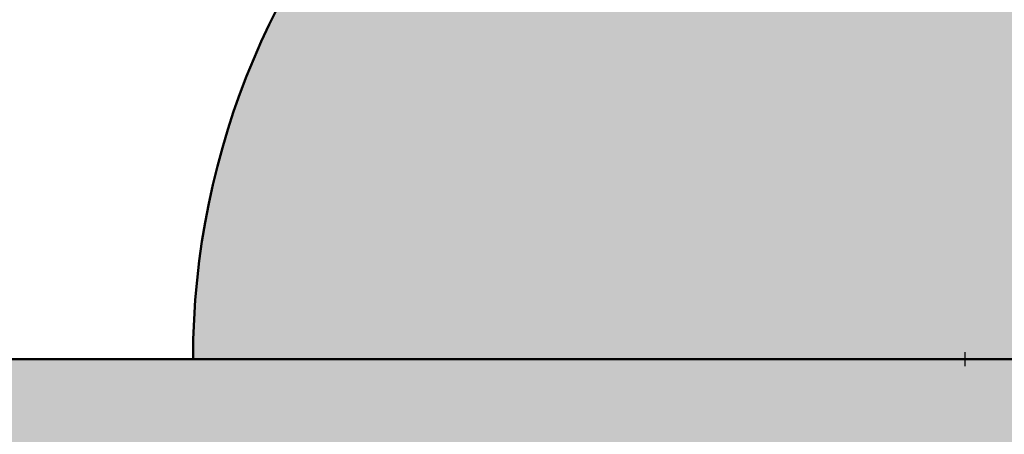
# Model space of a CAD drawing. Units: millimetres. Extents: x 0 to 2267, y 0 to 1823.
# Tile 14 of 256: x 1518.68 to 1531.44, y 1116.44 to 1121.82. Entities that reach past the tile are written whole.
import ezdxf

# ---------------------------------------------------------------- set-up
doc = ezdxf.new("R2010")
doc.units = ezdxf.units.MM
doc.header["$MEASUREMENT"] = 0
for name, color, linetype, lineweight in [('M-DIMS', 2, 'Continuous', 25), ('M-HATC', 252, 'Continuous', 18), ('M-OUTL', 7, 'Continuous', 50)]:
    doc.layers.add(name, color=color, linetype=linetype, lineweight=lineweight)
doc.styles.get("Standard").update_dxf_attribs({"font": 'arial.ttf'})
doc.dimstyles.get("Standard").update_dxf_attribs({"dimtxt": 7, "dimasz": 4, "dimexe": 0.18, "dimexo": 0.0625, "dimgap": 0.09, "dimtad": 0, "dimdec": 0, "dimzin": 0, "dimdsep": 46, "dimtxsty": 'Standard', "dimcen": 0.09, "dimadec": 0, "dimazin": 0, "dimtfac": 1, "dimtdec": 0, "dimtofl": 0, "dimtmove": 0, "dimatfit": 3, "dimfxl": 1, "dimtolj": 1, "dimtzin": 0, "dimarcsym": 0})

# ---------------------------------------------------------------- blocks, each defined once
blk = doc.blocks.new('*D28')
at = {"layer": 'Defpoints', "color": 0, "transparency": 16777216}
for p in [(1523.858, 1124.488), (1530.929, 1117.417)]:
    blk.add_point(p, dxfattribs=at)
at = {"layer": 'M-DIMS', "color": 0, "lineweight": -2, "transparency": 16777216}
for p, q in [((1518.201, 1130.145), (1521.029, 1127.317)), ((1530.839, 1117.417), (1531.019, 1117.417)), ((1530.929, 1117.327), (1530.929, 1117.507))]:
    blk.add_line(p, q, dxfattribs=at)
at = {"layer": 'M-DIMS', "color": 0, "transparency": 16777216}
blk.add_solid([(1521.501, 1127.788), (1520.558, 1126.845), (1523.858, 1124.488)], dxfattribs=at)
at = {"layer": 'M-DIMS', "color": 0, "transparency": 16777216, "insert": (1504.949, 1143.397), "char_height": 7, "attachment_point": 5, "rotation": 314.9998}
blk.add_mtext('\\A1;27X R10', dxfattribs=at)

msp = doc.modelspace()

# ---------------------------------------------------------------- hatches: boundary and pattern name
at = {"layer": 'M-HATC'}
h = msp.add_hatch(color=256, dxfattribs=at)
h.dxf.hatch_style = 1
h.paths.add_polyline_path([(2065.771, 1618.062, 0.236068), (2055.771, 1638.062), (1381.087, 1638.062, 0.236068), (1371.087, 1618.062), (1371.087, 1603.062), (2055.771, 1603.062), (2065.771, 1603.062)])
h.paths.add_polyline_path([(2062.772, 1550.296), (2062.772, 1560.296), (1374.086, 1560.296), (1374.086, 1550.296), (1374.086, 1540.296), (1384.086, 1540.296), (1389.086, 1540.296), (2062.772, 1540.296)])
h.paths.add_polyline_path([(1930.929, 1282.766), (1505.929, 1282.766), (1587.628, 1235.597, 0.131652), (1600.128, 1232.247), (1836.73, 1232.247, 0.131652), (1849.23, 1235.597)])
h.paths.add_polyline_path([(1930.929, 1117.417), (1905.929, 1117.417), (1505.929, 1117.417), (1505.929, 1077.417), (1930.929, 1077.417)])
h = msp.add_hatch(color=256, dxfattribs=at)
h.dxf.hatch_style = 1
h.paths.add_polyline_path([(2055.771, 1603.062), (1381.087, 1603.062), (1381.087, 1598.062), (2055.771, 1598.062)])
h.paths.add_polyline_path([(2055.771, 1598.062), (1381.087, 1598.062), (1381.087, 1593.062), (2055.771, 1593.062)])
h.paths.add_polyline_path([(2051.307, 1536.761), (1385.55, 1536.761), (1385.55, 1526.761), (1387.55, 1526.761), (1388.537, 1525.053), (1385.332, 1521.233), (1385.332, 1521.223), (2050.254, 1522.749), (2048.321, 1525.053), (2049.307, 1526.761), (2051.307, 1526.761)])
edge = h.paths.add_edge_path()
edge.add_arc((1847.535, 1379.149), 135, 222.60306, 222.89085, ccw=False)
edge.add_line((1748.166, 1287.766), (1683.092, 1287.766))
edge.add_arc((1583.724, 1379.149), 135, 317.10915, 317.39694, ccw=False)
edge.add_arc((1678.969, 1290.671), 5, 222.8909, 317.1091, ccw=False)
edge.add_arc((1774.213, 1379.149), 135, 222.60306, 222.89085, ccw=False)
edge.add_line((1674.845, 1287.766), (1609.771, 1287.766))
edge.add_arc((1510.403, 1379.149), 135, 317.10915, 317.39694, ccw=False)
edge.add_arc((1605.647, 1290.671), 5, 222.8909, 317.1091, ccw=False)
edge.add_arc((1700.892, 1379.149), 135, 222.60306, 222.89085, ccw=False)
edge.add_line((1601.524, 1287.766), (1536.45, 1287.766))
edge.add_arc((1437.081, 1379.149), 135, 317.10915, 317.39694, ccw=False)
edge.add_arc((1532.326, 1290.671), 5, 222.8909, 317.1091, ccw=False)
edge.add_arc((1627.571, 1379.149), 135, 222.60306, 222.89085, ccw=False)
edge.add_line((1528.203, 1287.766), (1505.929, 1287.766))
edge.add_spline(control_points=[(1505.929, 1287.766), (1504.262, 1287.766), (1504.262, 1282.766), (1505.929, 1282.766)], knot_values=[0, 0, 0, 0, 5, 5, 5, 5], degree=3, periodic=0)
edge.add_line((1505.929, 1282.766), (1930.929, 1282.766))
edge.add_spline(control_points=[(1930.929, 1282.766), (1932.596, 1282.766), (1932.596, 1287.766), (1930.929, 1287.766)], knot_values=[0, 0, 0, 0, 5, 5, 5, 5], degree=3, periodic=0)
edge.add_line((1930.929, 1287.766), (1903.056, 1287.766))
edge.add_arc((1803.688, 1379.149), 135, 317.10915, 317.39694, ccw=False)
edge.add_arc((1898.932, 1290.671), 5, 222.8909, 317.1091, ccw=False)
edge.add_arc((1994.177, 1379.149), 135, 222.60306, 222.89085, ccw=False)
edge.add_line((1894.809, 1287.766), (1829.735, 1287.766))
edge.add_arc((1730.366, 1379.149), 135, 317.10915, 317.39694, ccw=False)
edge.add_arc((1825.611, 1290.671), 5, 222.8909, 317.1091, ccw=False)
edge.add_arc((1920.856, 1379.149), 135, 222.60306, 222.89085, ccw=False)
edge.add_line((1821.487, 1287.766), (1756.413, 1287.766))
edge.add_arc((1657.045, 1379.149), 135, 317.10915, 317.39694, ccw=False)
edge.add_arc((1752.29, 1290.671), 5, 222.8909, 317.1091, ccw=False)
edge = h.paths.add_edge_path()
edge.add_spline(control_points=[(1843.429, 1227.247), (1845.096, 1227.247), (1845.096, 1232.247), (1843.429, 1232.247)], knot_values=[0, 0, 0, 0, 5, 5, 5, 5], degree=3, periodic=0)
edge.add_line((1843.429, 1232.247), (1593.429, 1232.247))
edge.add_spline(control_points=[(1593.429, 1232.247), (1591.762, 1232.247), (1591.762, 1227.247), (1593.429, 1227.247)], knot_values=[0, 0, 0, 0, 5, 5, 5, 5], degree=3, periodic=0)
edge.add_line((1593.429, 1227.247), (1843.429, 1227.247))
h.paths.add_polyline_path([(1905.929, 1127.417), (1530.929, 1127.417, 0.414214), (1520.929, 1117.417), (1530.929, 1117.417), (1915.929, 1117.417, 0.414214)])
edge = h.paths.add_edge_path()
edge.add_arc((1397.086, 1498.408), 12.73, 90.7821, 190.8787, ccw=False)
edge.add_line((1396.912, 1511.136), (1428.01, 1511.349))
edge.add_line((1428.01, 1511.349), (1433.01, 1511.349))
edge.add_line((1433.01, 1511.349), (1434.439, 1511.349))
edge.add_arc((1419.474, 1498.08), 20, 41.561, 74.0821)
edge.add_line((1424.959, 1517.314), (1399.935, 1517.256))
edge.add_spline(control_points=[(1399.931, 1517.256), (1399.884, 1517.213), (1399.833, 1517.169), (1399.777, 1517.124)], knot_values=[11.567499, 11.567499, 11.567499, 11.567499, 11.814249, 11.814249, 11.814249, 11.814249], degree=3, periodic=0)
edge.add_spline(control_points=[(1399.633, 1517.01), (1399.583, 1516.972), (1399.531, 1516.934), (1399.476, 1516.895)], knot_values=[11.167718, 11.167718, 11.167718, 11.167718, 11.365188, 11.365188, 11.365188, 11.365188], degree=3, periodic=0)
edge.add_spline(control_points=[(1399.34, 1516.8), (1399.151, 1516.672), (1398.938, 1516.538), (1398.704, 1516.399)], knot_values=[10.376405, 10.376405, 10.376405, 10.376405, 11.00994, 11.00994, 11.00994, 11.00994], degree=3, periodic=0)
edge.add_spline(control_points=[(1398.657, 1516.372), (1398.579, 1516.326), (1398.498, 1516.28), (1398.415, 1516.233)], knot_values=[10.125175, 10.125175, 10.125175, 10.125175, 10.334406, 10.334406, 10.334406, 10.334406], degree=3, periodic=0)
edge.add_spline(control_points=[(1398.264, 1516.149), (1398.196, 1516.111), (1398.126, 1516.073), (1398.055, 1516.035)], knot_values=[9.832246, 9.832246, 9.832246, 9.832246, 9.999658, 9.999658, 9.999658, 9.999658], degree=3, periodic=0)
edge.add_spline(control_points=[(1397.999, 1516.005), (1397.731, 1515.862), (1397.446, 1515.717), (1397.147, 1515.571)], knot_values=[9.161808, 9.161808, 9.161808, 9.161808, 9.787769, 9.787769, 9.787769, 9.787769], degree=3, periodic=0)
edge.add_spline(control_points=[(1397.147, 1515.571), (1396.842, 1515.423), (1396.522, 1515.274), (1396.191, 1515.126)], knot_values=[8.524455, 8.524455, 8.524455, 8.524455, 9.161808, 9.161808, 9.161808, 9.161808], degree=3, periodic=0)
edge.add_spline(control_points=[(1396.078, 1515.076), (1395.985, 1515.035), (1395.892, 1514.994), (1395.798, 1514.953)], knot_values=[8.275193, 8.275193, 8.275193, 8.275193, 8.451726, 8.451726, 8.451726, 8.451726], degree=3, periodic=0)
edge.add_spline(control_points=[(1395.602, 1514.869), (1395.5, 1514.826), (1395.397, 1514.782), (1395.293, 1514.739)], knot_values=[7.962917, 7.962917, 7.962917, 7.962917, 8.152764, 8.152764, 8.152764, 8.152764], degree=3, periodic=0)
edge.add_spline(control_points=[(1395.212, 1514.706), (1394.828, 1514.547), (1394.435, 1514.393), (1394.036, 1514.244)], knot_values=[7.21254, 7.21254, 7.21254, 7.21254, 7.913148, 7.913148, 7.913148, 7.913148], degree=3, periodic=0)
edge.add_spline(control_points=[(1394.036, 1514.244), (1393.708, 1514.121), (1393.375, 1514.003), (1393.043, 1513.889)], knot_values=[6.633733, 6.633733, 6.633733, 6.633733, 7.21254, 7.21254, 7.21254, 7.21254], degree=3, periodic=0)
edge.add_spline(control_points=[(1392.821, 1513.815), (1392.72, 1513.781), (1392.618, 1513.748), (1392.517, 1513.715)], knot_values=[6.328796, 6.328796, 6.328796, 6.328796, 6.505493, 6.505493, 6.505493, 6.505493], degree=3, periodic=0)
edge.add_spline(control_points=[(1392.517, 1513.715), (1392.319, 1513.652), (1392.121, 1513.59), (1391.924, 1513.531)], knot_values=[5.984605, 5.984605, 5.984605, 5.984605, 6.328796, 6.328796, 6.328796, 6.328796], degree=3, periodic=0)
edge.add_spline(control_points=[(1391.792, 1513.491), (1391.312, 1513.35), (1390.838, 1513.224), (1390.378, 1513.117)], knot_values=[5.066697, 5.066697, 5.066697, 5.066697, 5.907055, 5.907055, 5.907055, 5.907055], degree=3, periodic=0)
edge.add_spline(control_points=[(1390.378, 1513.117), (1390.18, 1513.071), (1389.984, 1513.028), (1389.791, 1512.99)], knot_values=[4.70367, 4.70367, 4.70367, 4.70367, 5.066695, 5.066695, 5.066695, 5.066695], degree=3, periodic=0)
edge.add_spline(control_points=[(1389.422, 1512.92), (1389.246, 1512.889), (1389.073, 1512.862), (1388.904, 1512.838)], knot_values=[4.130571, 4.130571, 4.130571, 4.130571, 4.469816, 4.469816, 4.469816, 4.469816], degree=3, periodic=0)
edge.add_spline(control_points=[(1388.904, 1512.838), (1388.591, 1512.795), (1388.291, 1512.764), (1388.007, 1512.749)], knot_values=[3.504031, 3.504031, 3.504031, 3.504031, 4.130571, 4.130571, 4.130571, 4.130571], degree=3, periodic=0)
edge.add_spline(control_points=[(1387.936, 1512.746), (1387.854, 1512.742), (1387.773, 1512.74), (1387.694, 1512.739)], knot_values=[3.268866, 3.268866, 3.268866, 3.268866, 3.451164, 3.451164, 3.451164, 3.451164], degree=3, periodic=0)
edge.add_spline(control_points=[(1387.335, 1512.744), (1387.208, 1512.75), (1387.085, 1512.76), (1386.967, 1512.774)], knot_values=[2.670686, 2.670686, 2.670686, 2.670686, 2.984, 2.984, 2.984, 2.984], degree=3, periodic=0)
edge.add_spline(control_points=[(1386.833, 1512.792), (1386.821, 1512.794), (1386.809, 1512.796), (1386.797, 1512.798)], knot_values=[2.516981, 2.516981, 2.516981, 2.516981, 2.549528, 2.549528, 2.549528, 2.549528], degree=3, periodic=0)
edge.add_spline(control_points=[(1386.453, 1512.873), (1386.426, 1512.881), (1386.399, 1512.889), (1386.373, 1512.897)], knot_values=[2.095869, 2.095869, 2.095869, 2.095869, 2.17941, 2.17941, 2.17941, 2.17941], degree=3, periodic=0)
edge.add_spline(control_points=[(1386.069, 1513.019), (1386.063, 1513.022), (1386.058, 1513.025), (1386.052, 1513.028)], knot_values=[1.72453, 1.72453, 1.72453, 1.72453, 1.745933, 1.745933, 1.745933, 1.745933], degree=3, periodic=0)
edge.add_arc((1399.474, 1498.08), 20, 131.8243, 180)
edge.add_arc((1630.334, 1505.548), 250.971, 181.70518, 236.42798)
edge.add_arc((1605.34, 1483.304), 218.782, 238.66083, 243.34961)
edge.add_arc((1647.091, 1510.359), 262.899, 183.12984, 237.85344, ccw=False)
h.paths.add_polyline_path([(1406.537, 1391.964, 0.149382), (1491.551, 1296.442, -0.129517)], flags=17)
edge = h.paths.add_edge_path()
edge.add_arc((2037.384, 1498.08), 20, 0, 48.2659)
edge.add_spline(control_points=[(2050.697, 1513.005), (2050.651, 1512.985), (2050.603, 1512.966), (2050.554, 1512.948)], knot_values=[1.835652, 1.835652, 1.835652, 1.835652, 2.000781, 2.000781, 2.000781, 2.000781], degree=3, periodic=0)
edge.add_spline(control_points=[(2050.462, 1512.917), (2050.479, 1512.922), (2050.496, 1512.928), (2050.513, 1512.934)], knot_values=[2.045477, 2.045477, 2.045477, 2.045477, 2.101389, 2.101389, 2.101389, 2.101389], degree=3, periodic=0)
edge.add_spline(control_points=[(2050.129, 1512.834), (2050.198, 1512.847), (2050.266, 1512.862), (2050.331, 1512.879)], knot_values=[2.237629, 2.237629, 2.237629, 2.237629, 2.435841, 2.435841, 2.435841, 2.435841], degree=3, periodic=0)
edge.add_spline(control_points=[(2050.095, 1512.828), (2050.106, 1512.83), (2050.118, 1512.832), (2050.129, 1512.834)], knot_values=[2.435841, 2.435841, 2.435841, 2.435841, 2.468321, 2.468321, 2.468321, 2.468321], degree=3, periodic=0)
edge.add_spline(control_points=[(2049.784, 1512.785), (2049.855, 1512.792), (2049.924, 1512.801), (2049.992, 1512.811)], knot_values=[2.563852, 2.563852, 2.563852, 2.563852, 2.748541, 2.748541, 2.748541, 2.748541], degree=3, periodic=0)
edge.add_spline(control_points=[(2049.405, 1512.762), (2049.536, 1512.765), (2049.663, 1512.773), (2049.784, 1512.785)], knot_values=[2.748541, 2.748541, 2.748541, 2.748541, 3.064882, 3.064882, 3.064882, 3.064882], degree=3, periodic=0)
edge.add_spline(control_points=[(2049.17, 1512.76), (2049.234, 1512.759), (2049.297, 1512.759), (2049.358, 1512.761)], knot_values=[3.102309, 3.102309, 3.102309, 3.102309, 3.2503, 3.2503, 3.2503, 3.2503], degree=3, periodic=0)
edge.add_spline(control_points=[(2048.857, 1512.769), (2048.964, 1512.764), (2049.068, 1512.761), (2049.17, 1512.76)], knot_values=[3.2503, 3.2503, 3.2503, 3.2503, 3.486069, 3.486069, 3.486069, 3.486069], degree=3, periodic=0)
edge.add_spline(control_points=[(2048.692, 1512.779), (2048.373, 1512.801), (2048.035, 1512.841), (2047.682, 1512.897)], knot_values=[3.606429, 3.606429, 3.606429, 3.606429, 4.2989, 4.2989, 4.2989, 4.2989], degree=3, periodic=0)
edge.add_spline(control_points=[(2047.682, 1512.897), (2047.546, 1512.919), (2047.408, 1512.942), (2047.268, 1512.969)], knot_values=[4.2989, 4.2989, 4.2989, 4.2989, 4.565769, 4.565769, 4.565769, 4.565769], degree=3, periodic=0)
edge.add_spline(control_points=[(2047.268, 1512.969), (2047.145, 1512.991), (2047.021, 1513.016), (2046.895, 1513.042)], knot_values=[4.565769, 4.565769, 4.565769, 4.565769, 4.799971, 4.799971, 4.799971, 4.799971], degree=3, periodic=0)
edge.add_spline(control_points=[(2046.895, 1513.042), (2046.529, 1513.119), (2046.151, 1513.209), (2045.768, 1513.311)], knot_values=[4.799971, 4.799971, 4.799971, 4.799971, 5.483718, 5.483718, 5.483718, 5.483718], degree=3, periodic=0)
edge.add_spline(control_points=[(2045.768, 1513.311), (2045.372, 1513.415), (2044.97, 1513.532), (2044.566, 1513.659)], knot_values=[5.483718, 5.483718, 5.483718, 5.483718, 6.187866, 6.187866, 6.187866, 6.187866], degree=3, periodic=0)
edge.add_spline(control_points=[(2044.566, 1513.659), (2044.415, 1513.706), (2044.263, 1513.755), (2044.112, 1513.805)], knot_values=[6.187866, 6.187866, 6.187866, 6.187866, 6.451551, 6.451551, 6.451551, 6.451551], degree=3, periodic=0)
edge.add_spline(control_points=[(2044.112, 1513.805), (2043.997, 1513.843), (2043.882, 1513.881), (2043.767, 1513.92)], knot_values=[6.451551, 6.451551, 6.451551, 6.451551, 6.651434, 6.651434, 6.651434, 6.651434], degree=3, periodic=0)
edge.add_spline(control_points=[(2043.767, 1513.92), (2043.372, 1514.055), (2042.977, 1514.198), (2042.589, 1514.346)], knot_values=[6.651434, 6.651434, 6.651434, 6.651434, 7.338879, 7.338879, 7.338879, 7.338879], degree=3, periodic=0)
edge.add_spline(control_points=[(2042.589, 1514.346), (2042.164, 1514.507), (2041.746, 1514.675), (2041.341, 1514.846)], knot_values=[7.338879, 7.338879, 7.338879, 7.338879, 8.089209, 8.089209, 8.089209, 8.089209], degree=3, periodic=0)
edge.add_spline(control_points=[(2041.341, 1514.846), (2041.103, 1514.946), (2040.869, 1515.048), (2040.64, 1515.15)], knot_values=[8.089209, 8.089209, 8.089209, 8.089209, 8.529587, 8.529587, 8.529587, 8.529587], degree=3, periodic=0)
edge.add_spline(control_points=[(2040.51, 1515.209), (2040.082, 1515.402), (2039.675, 1515.597), (2039.295, 1515.789)], knot_values=[8.613818, 8.613818, 8.613818, 8.613818, 9.44571, 9.44571, 9.44571, 9.44571], degree=3, periodic=0)
edge.add_spline(control_points=[(2039.295, 1515.789), (2039.062, 1515.907), (2038.839, 1516.025), (2038.629, 1516.14)], knot_values=[9.44571, 9.44571, 9.44571, 9.44571, 9.956404, 9.956404, 9.956404, 9.956404], degree=3, periodic=0)
edge.add_spline(control_points=[(2038.629, 1516.14), (2038.519, 1516.2), (2038.412, 1516.26), (2038.309, 1516.319)], knot_values=[9.956404, 9.956404, 9.956404, 9.956404, 10.223542, 10.223542, 10.223542, 10.223542], degree=3, periodic=0)
edge.add_spline(control_points=[(2038.309, 1516.319), (2038.214, 1516.374), (2038.122, 1516.428), (2038.033, 1516.481)], knot_values=[10.223542, 10.223542, 10.223542, 10.223542, 10.47051, 10.47051, 10.47051, 10.47051], degree=3, periodic=0)
edge.add_spline(control_points=[(2038.033, 1516.481), (2037.786, 1516.63), (2037.564, 1516.773), (2037.372, 1516.909)], knot_values=[10.47051, 10.47051, 10.47051, 10.47051, 11.15767, 11.15767, 11.15767, 11.15767], degree=3, periodic=0)
edge.add_spline(control_points=[(2037.372, 1516.909), (2037.279, 1516.975), (2037.193, 1517.04), (2037.114, 1517.102)], knot_values=[11.15767, 11.15767, 11.15767, 11.15767, 11.49227, 11.49227, 11.49227, 11.49227], degree=3, periodic=0)
edge.add_spline(control_points=[(2036.856, 1517.326), (2036.915, 1517.269), (2036.981, 1517.21), (2037.056, 1517.149)], knot_values=[11.577341, 11.577341, 11.577341, 11.577341, 11.91035, 11.91035, 11.91035, 11.91035], degree=3, periodic=0)
edge.add_spline(control_points=[(2036.807, 1517.375), (2036.823, 1517.359), (2036.839, 1517.342), (2036.856, 1517.326)], knot_values=[11.91035, 11.91035, 11.91035, 11.91035, 12.007402, 12.007402, 12.007402, 12.007402], degree=3, periodic=0)
edge.add_spline(control_points=[(2036.702, 1517.494), (2036.71, 1517.483), (2036.72, 1517.472), (2036.729, 1517.461)], knot_values=[12.184155, 12.184155, 12.184155, 12.184155, 12.255409, 12.255409, 12.255409, 12.255409], degree=3, periodic=0)
edge.add_spline(control_points=[(2036.616, 1517.621), (2036.62, 1517.613), (2036.624, 1517.606), (2036.629, 1517.598)], knot_values=[12.487913, 12.487913, 12.487913, 12.487913, 12.541035, 12.541035, 12.541035, 12.541035], degree=3, periodic=0)
edge.add_spline(control_points=[(2036.563, 1517.786), (2036.564, 1517.779), (2036.564, 1517.773), (2036.565, 1517.766)], knot_values=[12.911761, 12.911761, 12.911761, 12.911761, 12.968286, 12.968286, 12.968286, 12.968286], degree=3, periodic=0)
edge.add_spline(control_points=[(2036.617, 1517.93), (2036.612, 1517.926), (2036.609, 1517.921), (2036.605, 1517.916)], knot_values=[13.382527, 13.382527, 13.382527, 13.382527, 13.433791, 13.433791, 13.433791, 13.433791], degree=3, periodic=0)
edge.add_spline(control_points=[(2036.749, 1518.017), (2036.736, 1518.012), (2036.724, 1518.006), (2036.712, 1518)], knot_values=[13.726299, 13.726299, 13.726299, 13.726299, 13.809928, 13.809928, 13.809928, 13.809928], degree=3, periodic=0)
edge.add_spline(control_points=[(2036.86, 1518.053), (2036.839, 1518.047), (2036.818, 1518.042), (2036.799, 1518.035)], knot_values=[13.910887, 13.910887, 13.910887, 13.910887, 14.02153, 14.02153, 14.02153, 14.02153], degree=3, periodic=0)
edge.add_line((2036.964, 1518.08), (2032.384, 1518.08))
edge.add_line((2032.384, 1518.08), (2027.384, 1518.08))
edge.add_line((2027.384, 1518.08), (2022.384, 1518.08))
edge.add_line((2022.384, 1518.08), (2017.384, 1518.08))
edge.add_arc((2017.384, 1498.08), 20, 90, 138.439)
edge.add_line((2002.419, 1511.349), (2003.848, 1511.349))
edge.add_line((2003.848, 1511.349), (2008.848, 1511.349))
edge.add_line((2008.848, 1511.349), (2039.772, 1511.138))
edge.add_arc((2039.772, 1498.408), 12.73, -10.8787, 90, ccw=False)
edge.add_arc((1789.767, 1510.359), 262.899, 302.14656, 356.87016, ccw=False)
edge.add_arc((1831.518, 1483.304), 218.782, 296.65039, 301.33917)
edge.add_arc((1806.524, 1505.548), 250.971, 303.57202, 358.29482)
h.paths.add_polyline_path([(2030.321, 1391.964, -0.129517), (1945.307, 1296.442, 0.149382)], flags=17)
edge = h.paths.add_edge_path()
edge.add_spline(control_points=[(2037.246, 1518.082), (2037.29, 1518.081), (2037.336, 1518.08), (2037.384, 1518.08)], knot_values=[0.000012, 0.000012, 0.000012, 0.000012, 0.144754, 0.144754, 0.144754, 0.144754], degree=3, periodic=0)
edge.add_line((2037.336, 1518.08), (2037.01, 1518.08))
edge.add_spline(control_points=[(2037.01, 1518.08), (2036.982, 1518.077), (2036.956, 1518.073), (2036.931, 1518.068)], knot_values=[14.13465, 14.13465, 14.13465, 14.13465, 14.247197, 14.247197, 14.247197, 14.247197], degree=3, periodic=0)
edge.add_spline(control_points=[(2036.931, 1518.068), (2036.928, 1518.067), (2036.924, 1518.067), (2036.921, 1518.066)], knot_values=[14.118315, 14.118315, 14.118315, 14.118315, 14.13465, 14.13465, 14.13465, 14.13465], degree=3, periodic=0)
edge.add_spline(control_points=[(2036.921, 1518.066), (2036.912, 1518.064), (2036.903, 1518.063), (2036.895, 1518.061)], knot_values=[14.078086, 14.078086, 14.078086, 14.078086, 14.118315, 14.118315, 14.118315, 14.118315], degree=3, periodic=0)
edge.add_spline(control_points=[(2036.895, 1518.061), (2036.883, 1518.058), (2036.872, 1518.056), (2036.86, 1518.053)], knot_values=[14.02153, 14.02153, 14.02153, 14.02153, 14.078086, 14.078086, 14.078086, 14.078086], degree=3, periodic=0)
edge.add_spline(control_points=[(2036.86, 1518.053), (2036.839, 1518.047), (2036.818, 1518.042), (2036.799, 1518.035)], knot_values=[13.910887, 13.910887, 13.910887, 13.910887, 14.02153, 14.02153, 14.02153, 14.02153], degree=3, periodic=0)
edge.add_spline(control_points=[(2036.799, 1518.035), (2036.798, 1518.035), (2036.797, 1518.035), (2036.797, 1518.035)], knot_values=[13.906906, 13.906906, 13.906906, 13.906906, 13.910887, 13.910887, 13.910887, 13.910887], degree=3, periodic=0)
edge.add_spline(control_points=[(2036.797, 1518.035), (2036.788, 1518.032), (2036.78, 1518.029), (2036.772, 1518.026)], knot_values=[13.857826, 13.857826, 13.857826, 13.857826, 13.906906, 13.906906, 13.906906, 13.906906], degree=3, periodic=0)
edge.add_spline(control_points=[(2036.772, 1518.026), (2036.764, 1518.023), (2036.756, 1518.02), (2036.749, 1518.017)], knot_values=[13.809928, 13.809928, 13.809928, 13.809928, 13.857826, 13.857826, 13.857826, 13.857826], degree=3, periodic=0)
edge.add_spline(control_points=[(2036.749, 1518.017), (2036.736, 1518.012), (2036.724, 1518.006), (2036.712, 1518)], knot_values=[13.726299, 13.726299, 13.726299, 13.726299, 13.809928, 13.809928, 13.809928, 13.809928], degree=3, periodic=0)
edge.add_spline(control_points=[(2036.712, 1518), (2036.712, 1518), (2036.712, 1518), (2036.711, 1518)], knot_values=[13.723993, 13.723993, 13.723993, 13.723993, 13.726299, 13.726299, 13.726299, 13.726299], degree=3, periodic=0)
edge.add_spline(control_points=[(2036.711, 1518), (2036.706, 1517.997), (2036.701, 1517.994), (2036.696, 1517.992)], knot_values=[13.686536, 13.686536, 13.686536, 13.686536, 13.723993, 13.723993, 13.723993, 13.723993], degree=3, periodic=0)
edge.add_spline(control_points=[(2036.696, 1517.992), (2036.692, 1517.989), (2036.687, 1517.987), (2036.683, 1517.984)], knot_values=[13.651251, 13.651251, 13.651251, 13.651251, 13.686536, 13.686536, 13.686536, 13.686536], degree=3, periodic=0)
edge.add_spline(control_points=[(2036.683, 1517.984), (2036.676, 1517.98), (2036.67, 1517.976), (2036.664, 1517.971)], knot_values=[13.596804, 13.596804, 13.596804, 13.596804, 13.651251, 13.651251, 13.651251, 13.651251], degree=3, periodic=0)
edge.add_spline(control_points=[(2036.664, 1517.971), (2036.664, 1517.971), (2036.663, 1517.971), (2036.663, 1517.971)], knot_values=[13.593956, 13.593956, 13.593956, 13.593956, 13.596804, 13.596804, 13.596804, 13.596804], degree=3, periodic=0)
edge.add_spline(control_points=[(2036.663, 1517.971), (2036.66, 1517.969), (2036.658, 1517.967), (2036.655, 1517.965)], knot_values=[13.570322, 13.570322, 13.570322, 13.570322, 13.593956, 13.593956, 13.593956, 13.593956], degree=3, periodic=0)
edge.add_spline(control_points=[(2036.655, 1517.965), (2036.653, 1517.963), (2036.65, 1517.961), (2036.647, 1517.959)], knot_values=[13.545477, 13.545477, 13.545477, 13.545477, 13.570322, 13.570322, 13.570322, 13.570322], degree=3, periodic=0)
edge.add_spline(control_points=[(2036.647, 1517.959), (2036.647, 1517.959), (2036.647, 1517.959), (2036.647, 1517.959)], knot_values=[13.543931, 13.543931, 13.543931, 13.543931, 13.545477, 13.545477, 13.545477, 13.545477], degree=3, periodic=0)
edge.add_spline(control_points=[(2036.647, 1517.959), (2036.641, 1517.954), (2036.636, 1517.949), (2036.631, 1517.945)], knot_values=[13.488237, 13.488237, 13.488237, 13.488237, 13.543931, 13.543931, 13.543931, 13.543931], degree=3, periodic=0)
edge.add_spline(control_points=[(2036.631, 1517.945), (2036.628, 1517.942), (2036.626, 1517.94), (2036.623, 1517.937)], knot_values=[13.460307, 13.460307, 13.460307, 13.460307, 13.488237, 13.488237, 13.488237, 13.488237], degree=3, periodic=0)
edge.add_spline(control_points=[(2036.623, 1517.937), (2036.622, 1517.936), (2036.62, 1517.934), (2036.618, 1517.932)], knot_values=[13.439712, 13.439712, 13.439712, 13.439712, 13.460307, 13.460307, 13.460307, 13.460307], degree=3, periodic=0)
edge.add_spline(control_points=[(2036.618, 1517.932), (2036.618, 1517.931), (2036.617, 1517.931), (2036.617, 1517.93)], knot_values=[13.433791, 13.433791, 13.433791, 13.433791, 13.439712, 13.439712, 13.439712, 13.439712], degree=3, periodic=0)
edge.add_spline(control_points=[(2036.617, 1517.93), (2036.612, 1517.926), (2036.609, 1517.921), (2036.605, 1517.916)], knot_values=[13.382527, 13.382527, 13.382527, 13.382527, 13.433791, 13.433791, 13.433791, 13.433791], degree=3, periodic=0)
edge.add_spline(control_points=[(2036.605, 1517.916), (2036.603, 1517.913), (2036.6, 1517.91), (2036.598, 1517.907)], knot_values=[13.350017, 13.350017, 13.350017, 13.350017, 13.382527, 13.382527, 13.382527, 13.382527], degree=3, periodic=0)
edge.add_spline(control_points=[(2036.598, 1517.907), (2036.597, 1517.906), (2036.596, 1517.904), (2036.595, 1517.903)], knot_values=[13.333922, 13.333922, 13.333922, 13.333922, 13.350017, 13.350017, 13.350017, 13.350017], degree=3, periodic=0)
edge.add_spline(control_points=[(2036.595, 1517.903), (2036.595, 1517.902), (2036.594, 1517.901), (2036.593, 1517.9)], knot_values=[13.323828, 13.323828, 13.323828, 13.323828, 13.333922, 13.333922, 13.333922, 13.333922], degree=3, periodic=0)
edge.add_spline(control_points=[(2036.593, 1517.9), (2036.59, 1517.895), (2036.588, 1517.891), (2036.585, 1517.886)], knot_values=[13.277545, 13.277545, 13.277545, 13.277545, 13.323828, 13.323828, 13.323828, 13.323828], degree=3, periodic=0)
edge.add_spline(control_points=[(2036.585, 1517.886), (2036.584, 1517.883), (2036.582, 1517.879), (2036.58, 1517.875)], knot_values=[13.240119, 13.240119, 13.240119, 13.240119, 13.277545, 13.277545, 13.277545, 13.277545], degree=3, periodic=0)
edge.add_spline(control_points=[(2036.58, 1517.875), (2036.58, 1517.874), (2036.579, 1517.873), (2036.578, 1517.872)], knot_values=[13.228211, 13.228211, 13.228211, 13.228211, 13.240119, 13.240119, 13.240119, 13.240119], degree=3, periodic=0)
edge.add_spline(control_points=[(2036.578, 1517.872), (2036.578, 1517.87), (2036.577, 1517.869), (2036.577, 1517.868)], knot_values=[13.215717, 13.215717, 13.215717, 13.215717, 13.228211, 13.228211, 13.228211, 13.228211], degree=3, periodic=0)
edge.add_spline(control_points=[(2036.577, 1517.868), (2036.575, 1517.864), (2036.574, 1517.86), (2036.573, 1517.857)], knot_values=[13.179847, 13.179847, 13.179847, 13.179847, 13.215717, 13.215717, 13.215717, 13.215717], degree=3, periodic=0)
edge.add_spline(control_points=[(2036.573, 1517.857), (2036.571, 1517.851), (2036.57, 1517.846), (2036.569, 1517.841)], knot_values=[13.132017, 13.132017, 13.132017, 13.132017, 13.179847, 13.179847, 13.179847, 13.179847], degree=3, periodic=0)
edge.add_spline(control_points=[(2036.569, 1517.841), (2036.568, 1517.84), (2036.568, 1517.839), (2036.568, 1517.838)], knot_values=[13.122482, 13.122482, 13.122482, 13.122482, 13.132017, 13.132017, 13.132017, 13.132017], degree=3, periodic=0)
edge.add_spline(control_points=[(2036.568, 1517.838), (2036.568, 1517.836), (2036.567, 1517.835), (2036.567, 1517.833)], knot_values=[13.105592, 13.105592, 13.105592, 13.105592, 13.122482, 13.122482, 13.122482, 13.122482], degree=3, periodic=0)
edge.add_spline(control_points=[(2036.567, 1517.833), (2036.566, 1517.829), (2036.566, 1517.826), (2036.565, 1517.822)], knot_values=[13.074063, 13.074063, 13.074063, 13.074063, 13.105592, 13.105592, 13.105592, 13.105592], degree=3, periodic=0)
edge.add_spline(control_points=[(2036.565, 1517.822), (2036.565, 1517.822), (2036.565, 1517.822), (2036.565, 1517.822)], knot_values=[13.074043, 13.074043, 13.074043, 13.074043, 13.074063, 13.074063, 13.074063, 13.074063], degree=3, periodic=0)
edge.add_spline(control_points=[(2036.565, 1517.822), (2036.564, 1517.816), (2036.564, 1517.811), (2036.564, 1517.805)], knot_values=[13.021884, 13.021884, 13.021884, 13.021884, 13.074043, 13.074043, 13.074043, 13.074043], degree=3, periodic=0)
edge.add_spline(control_points=[(2036.564, 1517.805), (2036.564, 1517.804), (2036.564, 1517.803), (2036.564, 1517.803)], knot_values=[13.01674, 13.01674, 13.01674, 13.01674, 13.021884, 13.021884, 13.021884, 13.021884], degree=3, periodic=0)
edge.add_spline(control_points=[(2036.564, 1517.803), (2036.563, 1517.801), (2036.563, 1517.798), (2036.563, 1517.796)], knot_values=[12.996438, 12.996438, 12.996438, 12.996438, 13.01674, 13.01674, 13.01674, 13.01674], degree=3, periodic=0)
edge.add_spline(control_points=[(2036.563, 1517.796), (2036.563, 1517.793), (2036.563, 1517.789), (2036.563, 1517.786)], knot_values=[12.968286, 12.968286, 12.968286, 12.968286, 12.996438, 12.996438, 12.996438, 12.996438], degree=3, periodic=0)
edge.add_spline(control_points=[(2036.563, 1517.786), (2036.564, 1517.779), (2036.564, 1517.773), (2036.565, 1517.766)], knot_values=[12.911761, 12.911761, 12.911761, 12.911761, 12.968286, 12.968286, 12.968286, 12.968286], degree=3, periodic=0)
edge.add_spline(control_points=[(2036.565, 1517.766), (2036.565, 1517.766), (2036.565, 1517.766), (2036.565, 1517.766)], knot_values=[12.911017, 12.911017, 12.911017, 12.911017, 12.911761, 12.911761, 12.911761, 12.911761], degree=3, periodic=0)
edge.add_spline(control_points=[(2036.565, 1517.766), (2036.565, 1517.762), (2036.566, 1517.759), (2036.566, 1517.756)], knot_values=[12.88528, 12.88528, 12.88528, 12.88528, 12.911017, 12.911017, 12.911017, 12.911017], degree=3, periodic=0)
edge.add_spline(control_points=[(2036.566, 1517.756), (2036.567, 1517.753), (2036.567, 1517.751), (2036.568, 1517.748)], knot_values=[12.862519, 12.862519, 12.862519, 12.862519, 12.88528, 12.88528, 12.88528, 12.88528], degree=3, periodic=0)
edge.add_spline(control_points=[(2036.568, 1517.748), (2036.568, 1517.747), (2036.568, 1517.747), (2036.568, 1517.746)], knot_values=[12.858885, 12.858885, 12.858885, 12.858885, 12.862519, 12.862519, 12.862519, 12.862519], degree=3, periodic=0)
edge.add_spline(control_points=[(2036.568, 1517.746), (2036.569, 1517.74), (2036.571, 1517.733), (2036.572, 1517.726)], knot_values=[12.8053, 12.8053, 12.8053, 12.8053, 12.858885, 12.858885, 12.858885, 12.858885], degree=3, periodic=0)
edge.add_spline(control_points=[(2036.572, 1517.726), (2036.573, 1517.723), (2036.574, 1517.719), (2036.576, 1517.715)], knot_values=[12.775176, 12.775176, 12.775176, 12.775176, 12.8053, 12.8053, 12.8053, 12.8053], degree=3, periodic=0)
edge.add_spline(control_points=[(2036.576, 1517.715), (2036.576, 1517.713), (2036.577, 1517.71), (2036.578, 1517.708)], knot_values=[12.756759, 12.756759, 12.756759, 12.756759, 12.775176, 12.775176, 12.775176, 12.775176], degree=3, periodic=0)
edge.add_spline(control_points=[(2036.578, 1517.708), (2036.578, 1517.707), (2036.578, 1517.706), (2036.579, 1517.705)], knot_values=[12.748742, 12.748742, 12.748742, 12.748742, 12.756759, 12.756759, 12.756759, 12.756759], degree=3, periodic=0)
edge.add_spline(control_points=[(2036.579, 1517.705), (2036.581, 1517.698), (2036.583, 1517.692), (2036.586, 1517.685)], knot_values=[12.69959, 12.69959, 12.69959, 12.69959, 12.748742, 12.748742, 12.748742, 12.748742], degree=3, periodic=0)
edge.add_spline(control_points=[(2036.586, 1517.685), (2036.588, 1517.68), (2036.59, 1517.675), (2036.592, 1517.669)], knot_values=[12.659038, 12.659038, 12.659038, 12.659038, 12.69959, 12.69959, 12.69959, 12.69959], degree=3, periodic=0)
edge.add_spline(control_points=[(2036.592, 1517.669), (2036.594, 1517.665), (2036.596, 1517.66), (2036.598, 1517.656)], knot_values=[12.626806, 12.626806, 12.626806, 12.626806, 12.659038, 12.659038, 12.659038, 12.659038], degree=3, periodic=0)
edge.add_spline(control_points=[(2036.598, 1517.656), (2036.598, 1517.655), (2036.599, 1517.654), (2036.599, 1517.653)], knot_values=[12.619394, 12.619394, 12.619394, 12.619394, 12.626806, 12.626806, 12.626806, 12.626806], degree=3, periodic=0)
edge.add_spline(control_points=[(2036.599, 1517.653), (2036.604, 1517.642), (2036.61, 1517.632), (2036.616, 1517.621)], knot_values=[12.541039, 12.541039, 12.541039, 12.541039, 12.619394, 12.619394, 12.619394, 12.619394], degree=3, periodic=0)
edge.add_spline(control_points=[(2036.616, 1517.621), (2036.616, 1517.621), (2036.616, 1517.621), (2036.616, 1517.621)], knot_values=[12.541035, 12.541035, 12.541035, 12.541035, 12.541039, 12.541039, 12.541039, 12.541039], degree=3, periodic=0)
edge.add_spline(control_points=[(2036.616, 1517.621), (2036.62, 1517.613), (2036.624, 1517.606), (2036.629, 1517.598)], knot_values=[12.487913, 12.487913, 12.487913, 12.487913, 12.541035, 12.541035, 12.541035, 12.541035], degree=3, periodic=0)
edge.add_spline(control_points=[(2036.629, 1517.598), (2036.633, 1517.592), (2036.637, 1517.585), (2036.641, 1517.579)], knot_values=[12.443982, 12.443982, 12.443982, 12.443982, 12.487913, 12.487913, 12.487913, 12.487913], degree=3, periodic=0)
edge.add_spline(control_points=[(2036.641, 1517.579), (2036.641, 1517.578), (2036.642, 1517.576), (2036.643, 1517.575)], knot_values=[12.434996, 12.434996, 12.434996, 12.434996, 12.443982, 12.443982, 12.443982, 12.443982], degree=3, periodic=0)
edge.add_spline(control_points=[(2036.643, 1517.575), (2036.653, 1517.56), (2036.664, 1517.544), (2036.676, 1517.528)], knot_values=[12.329647, 12.329647, 12.329647, 12.329647, 12.434996, 12.434996, 12.434996, 12.434996], degree=3, periodic=0)
edge.add_spline(control_points=[(2036.676, 1517.528), (2036.684, 1517.517), (2036.693, 1517.505), (2036.702, 1517.494)], knot_values=[12.255409, 12.255409, 12.255409, 12.255409, 12.329647, 12.329647, 12.329647, 12.329647], degree=3, periodic=0)
edge.add_spline(control_points=[(2036.702, 1517.494), (2036.71, 1517.483), (2036.72, 1517.472), (2036.729, 1517.461)], knot_values=[12.184155, 12.184155, 12.184155, 12.184155, 12.255409, 12.255409, 12.255409, 12.255409], degree=3, periodic=0)
edge.add_spline(control_points=[(2036.729, 1517.461), (2036.744, 1517.444), (2036.759, 1517.426), (2036.775, 1517.409)], knot_values=[12.075961, 12.075961, 12.075961, 12.075961, 12.184155, 12.184155, 12.184155, 12.184155], degree=3, periodic=0)
edge.add_spline(control_points=[(2036.775, 1517.409), (2036.776, 1517.407), (2036.777, 1517.406), (2036.778, 1517.405)], knot_values=[12.069502, 12.069502, 12.069502, 12.069502, 12.075961, 12.075961, 12.075961, 12.075961], degree=3, periodic=0)
edge.add_spline(control_points=[(2036.778, 1517.405), (2036.788, 1517.395), (2036.797, 1517.385), (2036.807, 1517.375)], knot_values=[12.007402, 12.007402, 12.007402, 12.007402, 12.069502, 12.069502, 12.069502, 12.069502], degree=3, periodic=0)
edge.add_spline(control_points=[(2036.807, 1517.375), (2036.823, 1517.359), (2036.839, 1517.342), (2036.856, 1517.326)], knot_values=[11.91035, 11.91035, 11.91035, 11.91035, 12.007402, 12.007402, 12.007402, 12.007402], degree=3, periodic=0)
edge.add_spline(control_points=[(2036.856, 1517.326), (2036.915, 1517.269), (2036.981, 1517.21), (2037.056, 1517.149)], knot_values=[11.577341, 11.577341, 11.577341, 11.577341, 11.91035, 11.91035, 11.91035, 11.91035], degree=3, periodic=0)
edge.add_spline(control_points=[(2037.056, 1517.149), (2037.075, 1517.134), (2037.094, 1517.118), (2037.114, 1517.102)], knot_values=[11.49227, 11.49227, 11.49227, 11.49227, 11.577341, 11.577341, 11.577341, 11.577341], degree=3, periodic=0)
edge.add_spline(control_points=[(2037.114, 1517.102), (2037.193, 1517.04), (2037.279, 1516.975), (2037.372, 1516.909)], knot_values=[11.15767, 11.15767, 11.15767, 11.15767, 11.49227, 11.49227, 11.49227, 11.49227], degree=3, periodic=0)
edge.add_spline(control_points=[(2037.372, 1516.909), (2037.564, 1516.773), (2037.786, 1516.63), (2038.033, 1516.481)], knot_values=[10.47051, 10.47051, 10.47051, 10.47051, 11.15767, 11.15767, 11.15767, 11.15767], degree=3, periodic=0)
edge.add_spline(control_points=[(2038.033, 1516.481), (2038.122, 1516.428), (2038.214, 1516.374), (2038.309, 1516.319)], knot_values=[10.223542, 10.223542, 10.223542, 10.223542, 10.47051, 10.47051, 10.47051, 10.47051], degree=3, periodic=0)
edge.add_spline(control_points=[(2038.309, 1516.319), (2038.412, 1516.26), (2038.519, 1516.2), (2038.629, 1516.14)], knot_values=[9.956404, 9.956404, 9.956404, 9.956404, 10.223542, 10.223542, 10.223542, 10.223542], degree=3, periodic=0)
edge.add_spline(control_points=[(2038.629, 1516.14), (2038.839, 1516.025), (2039.062, 1515.907), (2039.295, 1515.789)], knot_values=[9.44571, 9.44571, 9.44571, 9.44571, 9.956404, 9.956404, 9.956404, 9.956404], degree=3, periodic=0)
edge.add_spline(control_points=[(2039.295, 1515.789), (2039.675, 1515.597), (2040.082, 1515.402), (2040.51, 1515.209)], knot_values=[8.613818, 8.613818, 8.613818, 8.613818, 9.44571, 9.44571, 9.44571, 9.44571], degree=3, periodic=0)
edge.add_spline(control_points=[(2040.51, 1515.209), (2040.553, 1515.189), (2040.597, 1515.17), (2040.64, 1515.15)], knot_values=[8.529587, 8.529587, 8.529587, 8.529587, 8.613818, 8.613818, 8.613818, 8.613818], degree=3, periodic=0)
edge.add_spline(control_points=[(2040.64, 1515.15), (2040.869, 1515.048), (2041.103, 1514.946), (2041.341, 1514.846)], knot_values=[8.089209, 8.089209, 8.089209, 8.089209, 8.529587, 8.529587, 8.529587, 8.529587], degree=3, periodic=0)
edge.add_spline(control_points=[(2041.341, 1514.846), (2041.746, 1514.675), (2042.164, 1514.507), (2042.589, 1514.346)], knot_values=[7.338879, 7.338879, 7.338879, 7.338879, 8.089209, 8.089209, 8.089209, 8.089209], degree=3, periodic=0)
edge.add_spline(control_points=[(2042.589, 1514.346), (2042.977, 1514.198), (2043.372, 1514.055), (2043.767, 1513.92)], knot_values=[6.651434, 6.651434, 6.651434, 6.651434, 7.338879, 7.338879, 7.338879, 7.338879], degree=3, periodic=0)
edge.add_spline(control_points=[(2043.767, 1513.92), (2043.882, 1513.881), (2043.997, 1513.843), (2044.112, 1513.805)], knot_values=[6.451551, 6.451551, 6.451551, 6.451551, 6.651434, 6.651434, 6.651434, 6.651434], degree=3, periodic=0)
edge.add_spline(control_points=[(2044.112, 1513.805), (2044.263, 1513.755), (2044.415, 1513.706), (2044.566, 1513.659)], knot_values=[6.187866, 6.187866, 6.187866, 6.187866, 6.451551, 6.451551, 6.451551, 6.451551], degree=3, periodic=0)
edge.add_spline(control_points=[(2044.566, 1513.659), (2044.97, 1513.532), (2045.372, 1513.415), (2045.768, 1513.311)], knot_values=[5.483718, 5.483718, 5.483718, 5.483718, 6.187866, 6.187866, 6.187866, 6.187866], degree=3, periodic=0)
edge.add_spline(control_points=[(2045.768, 1513.311), (2046.151, 1513.209), (2046.529, 1513.119), (2046.895, 1513.042)], knot_values=[4.799971, 4.799971, 4.799971, 4.799971, 5.483718, 5.483718, 5.483718, 5.483718], degree=3, periodic=0)
edge.add_spline(control_points=[(2046.895, 1513.042), (2047.021, 1513.016), (2047.145, 1512.991), (2047.268, 1512.969)], knot_values=[4.565769, 4.565769, 4.565769, 4.565769, 4.799971, 4.799971, 4.799971, 4.799971], degree=3, periodic=0)
edge.add_spline(control_points=[(2047.268, 1512.969), (2047.408, 1512.942), (2047.546, 1512.919), (2047.682, 1512.897)], knot_values=[4.2989, 4.2989, 4.2989, 4.2989, 4.565769, 4.565769, 4.565769, 4.565769], degree=3, periodic=0)
edge.add_spline(control_points=[(2047.682, 1512.897), (2048.035, 1512.841), (2048.373, 1512.801), (2048.692, 1512.779)], knot_values=[3.606429, 3.606429, 3.606429, 3.606429, 4.2989, 4.2989, 4.2989, 4.2989], degree=3, periodic=0)
edge.add_spline(control_points=[(2048.692, 1512.779), (2048.748, 1512.775), (2048.803, 1512.772), (2048.857, 1512.769)], knot_values=[3.486069, 3.486069, 3.486069, 3.486069, 3.606429, 3.606429, 3.606429, 3.606429], degree=3, periodic=0)
edge.add_spline(control_points=[(2048.857, 1512.769), (2048.964, 1512.764), (2049.068, 1512.761), (2049.17, 1512.76)], knot_values=[3.2503, 3.2503, 3.2503, 3.2503, 3.486069, 3.486069, 3.486069, 3.486069], degree=3, periodic=0)
edge.add_spline(control_points=[(2049.17, 1512.76), (2049.234, 1512.759), (2049.297, 1512.759), (2049.358, 1512.761)], knot_values=[3.102309, 3.102309, 3.102309, 3.102309, 3.2503, 3.2503, 3.2503, 3.2503], degree=3, periodic=0)
edge.add_spline(control_points=[(2049.358, 1512.761), (2049.374, 1512.761), (2049.39, 1512.761), (2049.405, 1512.762)], knot_values=[3.064882, 3.064882, 3.064882, 3.064882, 3.102309, 3.102309, 3.102309, 3.102309], degree=3, periodic=0)
edge.add_spline(control_points=[(2049.405, 1512.762), (2049.536, 1512.765), (2049.663, 1512.773), (2049.784, 1512.785)], knot_values=[2.748541, 2.748541, 2.748541, 2.748541, 3.064882, 3.064882, 3.064882, 3.064882], degree=3, periodic=0)
edge.add_spline(control_points=[(2049.784, 1512.785), (2049.855, 1512.792), (2049.924, 1512.801), (2049.992, 1512.811)], knot_values=[2.563852, 2.563852, 2.563852, 2.563852, 2.748541, 2.748541, 2.748541, 2.748541], degree=3, periodic=0)
edge.add_spline(control_points=[(2049.992, 1512.811), (2050.026, 1512.816), (2050.061, 1512.822), (2050.095, 1512.828)], knot_values=[2.468321, 2.468321, 2.468321, 2.468321, 2.563852, 2.563852, 2.563852, 2.563852], degree=3, periodic=0)
edge.add_spline(control_points=[(2050.095, 1512.828), (2050.106, 1512.83), (2050.118, 1512.832), (2050.129, 1512.834)], knot_values=[2.435841, 2.435841, 2.435841, 2.435841, 2.468321, 2.468321, 2.468321, 2.468321], degree=3, periodic=0)
edge.add_spline(control_points=[(2050.129, 1512.834), (2050.198, 1512.847), (2050.266, 1512.862), (2050.331, 1512.879)], knot_values=[2.237629, 2.237629, 2.237629, 2.237629, 2.435841, 2.435841, 2.435841, 2.435841], degree=3, periodic=0)
edge.add_spline(control_points=[(2050.331, 1512.879), (2050.375, 1512.891), (2050.419, 1512.903), (2050.462, 1512.917)], knot_values=[2.101389, 2.101389, 2.101389, 2.101389, 2.237629, 2.237629, 2.237629, 2.237629], degree=3, periodic=0)
edge.add_spline(control_points=[(2050.462, 1512.917), (2050.479, 1512.922), (2050.496, 1512.928), (2050.513, 1512.934)], knot_values=[2.045477, 2.045477, 2.045477, 2.045477, 2.101389, 2.101389, 2.101389, 2.101389], degree=3, periodic=0)
edge.add_spline(control_points=[(2050.513, 1512.934), (2050.527, 1512.938), (2050.54, 1512.943), (2050.554, 1512.948)], knot_values=[2.000781, 2.000781, 2.000781, 2.000781, 2.045477, 2.045477, 2.045477, 2.045477], degree=3, periodic=0)
edge.add_spline(control_points=[(2050.554, 1512.948), (2050.603, 1512.966), (2050.651, 1512.985), (2050.697, 1513.005)], knot_values=[1.835652, 1.835652, 1.835652, 1.835652, 2.000781, 2.000781, 2.000781, 2.000781], degree=3, periodic=0)
edge.add_arc((2037.384, 1498.08), 20, 48.2659, 90.1299)
edge = h.paths.add_edge_path(flags=16)
edge.add_spline(control_points=[(1386.139, 1512.986), (1388.92, 1511.739), (1398.039, 1515.519), (1399.931, 1517.256)], knot_values=[1.831046, 1.831046, 1.831046, 1.831046, 11.814249, 11.814249, 11.814249, 11.814249], degree=3, periodic=0)
edge.add_line((1399.931, 1517.256), (1393.743, 1517.242))
edge.add_arc((1399.474, 1498.08), 20, 106.6501, 131.8173)

# ---------------------------------------------------------------- linework, layer by layer
at = {"layer": 'M-OUTL'}
for p, q in [((1505.929, 1117.417), (1930.929, 1117.417)), ((1505.929, 1117.417), (1530.929, 1117.417)), ((1530.929, 1117.417), (1520.929, 1117.417))]:
    msp.add_line(p, q, dxfattribs=at)
msp.add_arc((1530.929, 1117.417), 10, 90, 180, dxfattribs=at)

# ---------------------------------------------------------------- dimensions: what is measured, and where the dimension line sits
at = {"layer": 'M-DIMS'}
dim = msp.add_radius_dim(center=(1530.929, 1117.417), mpoint=(1523.858, 1124.488), text='27X <>', dimstyle='Standard', override={"dimdec": 0, "dimlfac": 1, "dimrnd": 0, "dimzin": 0, "dimdsep": 46, "dimlunit": 2}, dxfattribs=at)
dim.commit()
dim.dimension.update_dxf_attribs({"geometry": '*D28', "text_midpoint": (1504.949, 1143.397)})

doc.saveas('drawing.dxf')
